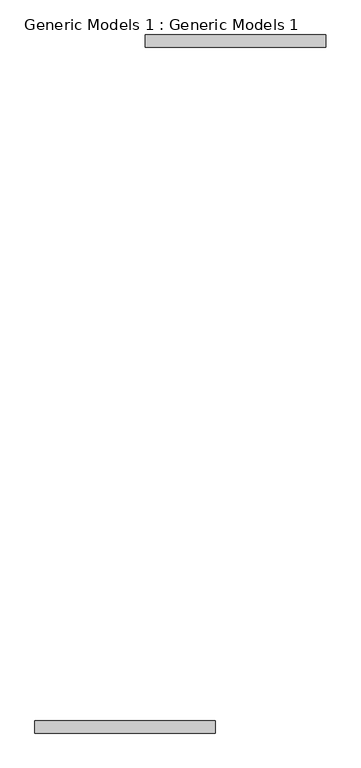
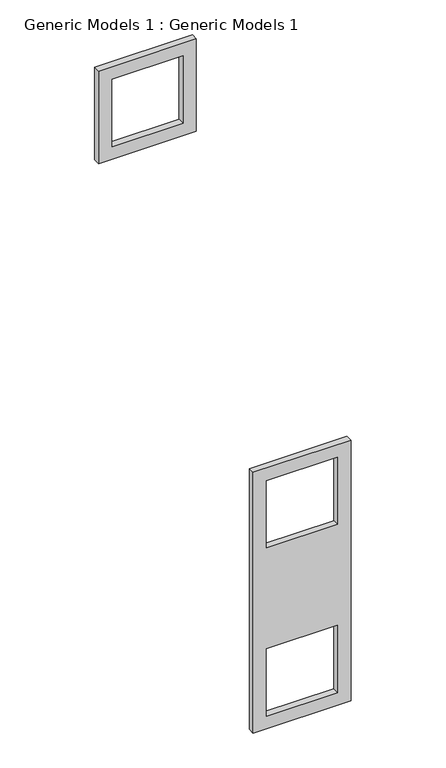
"""IFC4 building model written with IfcOpenShell, lengths in millimetres: proxy geometry, Generic Models 1 : Generic Models 1."""

from ifc_helpers import new_model, si_unit, frame, origin, place, context, project, spatial, polyline, outline, extrude, source, transform, mapped, element, save


def generic_models_1_generic_models_1_5e281b0c(model_context):
    return source(origin(), model_context, "Body", "SweptSolid", [
        extrude(outline(polyline([(8458.2, -66.5608498), (8458.2, -1742.9608498), (6781.8, -1742.9608498), (6781.8, -66.5608498), (8458.2, -66.5608498)]), holes=[polyline([(8229.6, -295.1608498), (7010.4, -295.1608498), (7010.4, -1514.3608498), (8229.6, -1514.3608498), (8229.6, -295.1608498)])]), frame((0.0, 923.7115866, 0.0), z_axis=(0.0, 1.0, 0.0), x_axis=(0.0, 0.0, 1.0)), (0.0, 0.0, 1.0), 114.3),
        extrude(outline(polyline([(685.8, -2770.9608498), (685.8, -1094.5608498), (5410.2, -1094.5608498), (5410.2, -2770.9608498), (685.8, -2770.9608498)]), holes=[polyline([(5181.6, -1323.1608498), (3962.4, -1323.1608498), (3962.4, -2542.3608498), (5181.6, -2542.3608498), (5181.6, -1323.1608498)]), polyline([(2133.6, -2542.3608498), (2133.6, -1323.1608498), (914.4, -1323.1608498), (914.4, -2542.3608498), (2133.6, -2542.3608498)])]), frame((0.0, -5452.3884134, 0.0), z_axis=(0.0, 1.0, 0.0), x_axis=(0.0, 0.0, 1.0)), (0.0, 0.0, 1.0), 114.3),
    ])


if __name__ == "__main__":
    model = new_model("IFC4")
    model_context = context("Model", 3, world=origin())
    ifc_project = project(units=[si_unit("LENGTHUNIT", "METRE", prefix="MILLI")], contexts=[model_context])
    site = spatial("IfcSite", under=ifc_project)
    building = spatial("IfcBuilding", under=site)
    placement = place(None, origin())
    generic_models_1_generic_models_1_shape = generic_models_1_generic_models_1_5e281b0c(model_context)
    element("IfcBuildingElementProxy", 1, Name="Generic Models 1 : Generic Models 1", ObjectType="Generic Models 1 : Generic Models 1", at=placement, inside=building, context=model_context, shape_type="MappedRepresentation", body=[
        mapped(generic_models_1_generic_models_1_shape, transform((0.0, 0.0, 0.0), x_axis=(1.0, 0.0, 0.0), y_axis=(0.0, 1.0, 0.0), z_axis=(0.0, 0.0, 1.0))),
    ])
    save(model, "model.ifc")

# Revit data of these elements
# Element 1 (IfcBuildingElementProxy, "Generic Models 1 : Generic Models 1")
#   Materials on its faces: "white colour"
# Materials
#   "white colour": class "Generic", colour RGB 120 120 120, transparency 0, Cost = 0
